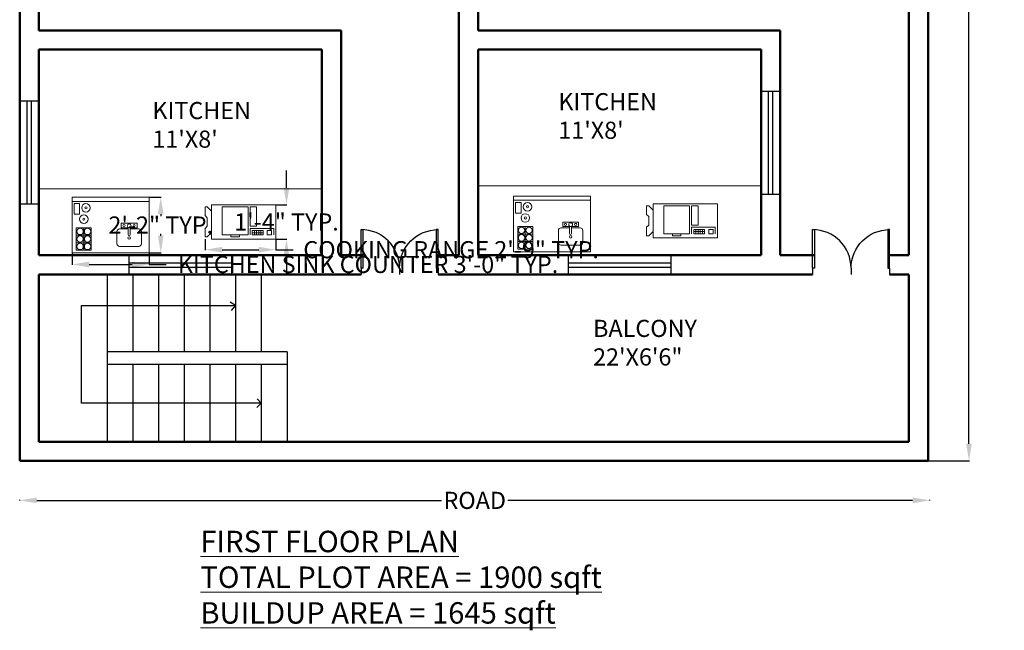
# Model space of a CAD drawing. Units: inches. Extents: x 179 to 2009, y 628 to 2084.
# Tile 3 of 5: x 766 to 1226, y 1391 to 1676. Entities that reach past the tile are written whole.
import ezdxf

# ---------------------------------------------------------------- set-up
doc = ezdxf.new("R2010")
doc.units = ezdxf.units.IN
doc.header["$MEASUREMENT"] = 0
for name, color, linetype, lineweight in [('A-ANNO-DIMS', 2, 'Continuous', 18), ('A-ANNO-TEXT', 7, 'Continuous', 18), ('A-DOOR', 3, 'Continuous', 25), ('A-FLOR-STRS', 6, 'Continuous', 25), ('A-FURN', 4, 'Continuous', 18), ('A-GLAZ', 2, 'Continuous', 25), ('A-WALL', 1, 'Continuous', 50)]:
    doc.layers.add(name, color=color, linetype=linetype, lineweight=lineweight)
doc.styles.get("Standard").update_dxf_attribs({"font": 'arial.ttf'})
doc.dimstyles.get("Standard").update_dxf_attribs({"dimtxt": 8, "dimasz": 8, "dimexe": 0.18, "dimexo": 0.0625, "dimgap": 0.09, "dimtad": 0, "dimtih": 1, "dimtoh": 1, "dimdec": 0, "dimzin": 0, "dimdsep": 46, "dimlunit": 3, "dimtxsty": 'Standard', "dimcen": 0.09, "dimadec": 0, "dimazin": 0, "dimtfac": 1, "dimtdec": 0, "dimtofl": 0, "dimtmove": 0, "dimatfit": 3, "dimfxl": 1, "dimtolj": 1, "dimtzin": 0, "dimarcsym": 0})

# ---------------------------------------------------------------- blocks, each defined once
blk = doc.blocks.new('*U4')
for p, q in [((0, 0), (0, -6)), ((36, 0), (36, -6))]:
    blk.add_line(p, q)
blk.add_lwpolyline([(0, 0), (0, 36), (1.75, 36), (1.75, 0)], close=True)
blk.add_arc((0, 0), 36, 0, 90)
blk = doc.blocks.new('Wet Bar')
for p, q in [((0, 0), (36, 0)), ((0, -26), (0, 0)), ((36, 0), (36, -26)), ((0, -2), (36, -2)), ((3.5, -3), (1, -3)), ((1, -3), (1, -8)), ((3.5, -8), (3.5, -3)), ((1, -8), (3.5, -8)), ((2, -14.25), (9, -14.25)), ((2, -24.75), (2, -14.25)), ((2, -17.75), (9, -17.75)), ((5.5, -14.25), (5.5, -24.75)), ((9, -14.25), (9, -24.75)), ((26.2, -17.55), (26.2, -14.1284)), ((27.1001, -17.55), (27.1001, -14.1284)), ((9, -21.25), (2, -21.25)), ((36, -26), (0, -26)), ((9, -24.75), (2, -24.75))]:
    blk.add_line(p, q)
for points in [[(26.2, -14.25), (22.95, -14.25), (22.95, -12.2), (26.75, -12.2)], [(26.7487, -12.2), (30.3501, -12.2), (30.3501, -14.25), (27.1001, -14.25)], [(20.95, -21.75), (20.95, -16.05)], [(22.15, -14.85), (26.2, -14.85)], [(27.1001, -14.85), (31.15, -14.85)], [(32.3501, -16.05), (32.3501, -21.75)], [(31.15, -22.95), (22.15, -22.95)]]:
    blk.add_lwpolyline(points)
for centre, radius in [((6.5, -5), 2), ((6.5, -5), 0.5), ((5.5, -10.25), 2), ((5.5, -10.25), 0.5), ((24.25, -13.25), 0.5), ((26.65, -13.35), 0.9), ((29, -13.25), 0.5), ((3.75, -16), 1.5), ((3.75, -19.5), 1.5), ((7.25, -16), 1.5), ((7.25, -19.5), 1.5), ((3.75, -23), 1.5), ((7.25, -23), 1.5), ((26.65, -19.05), 0.6)]:
    blk.add_circle(centre, radius)
for centre, radius, start, end in [((22.2251, -16.125), 1.2772, 93.36646, 176.6335), ((26.65, -17.55), 0.45, 180, 0), ((31.075, -16.125), 1.2772, 3.366461, 86.63354), ((22.2251, -21.675), 1.2772, 183.3665, 266.6335), ((31.075, -21.675), 1.2772, 273.3665, 356.6335)]:
    blk.add_arc(centre, radius, start, end)
blk = doc.blocks.new('Copy Machine')
for p, q in [((0, 0), (0, -16)), ((30, 0), (0, 0)), ((30, -16), (30, 0)), ((-3, -1), (-3, -5)), ((-2, -1), (-3, -1)), ((0, -3), (-2, -1)), ((5, -1), (5, -14)), ((17, -1), (5, -1)), ((17, -14), (17, -1)), ((18, -1), (18, -10)), ((21, -1), (18, -1)), ((21, -10), (21, -1)), ((-3, -5), (-2, -6)), ((-2, -10), (-2, -6)), ((-3, -11), (-2, -10)), ((-3, -15), (-3, -11)), ((0, -13), (-2, -15)), ((18, -10), (21, -10)), ((18, -14), (18, -11)), ((18, -11), (29, -11)), ((24, -12), (19, -12)), ((19, -12), (19, -14)), ((24, -13), (19, -13)), ((20, -12), (20, -14)), ((21, -14), (21, -12)), ((22, -12), (22, -14)), ((23, -14), (23, -12)), ((24, -14), (24, -12)), ((28, -12), (26, -12)), ((26, -12), (26, -14)), ((28, -14), (28, -12)), ((29, -11), (29, -14)), ((-2, -15), (-3, -15)), ((0, -16), (30, -16)), ((5, -14), (17, -14)), ((9, -14), (9, -15)), ((9, -15), (13, -15)), ((13, -15), (13, -14)), ((19, -14), (24, -14)), ((26, -14), (28, -14))]:
    blk.add_line(p, q)
blk = doc.blocks.new('*D18')
at = {"layer": 'A-ANNO-DIMS', "color": 0, "lineweight": -2, "transparency": 16777216}
for p, q in [((1190.56, 2043.18), (1209.72, 2043.18)), ((1209.54, 2035.18), (1209.54, 1760.86)), ((1209.54, 1478.18), (1209.54, 1752.51)), ((1190.56, 1470.18), (1209.72, 1470.18))]:
    blk.add_line(p, q, dxfattribs=at)
at = {"layer": 'A-ANNO-DIMS', "color": 0, "transparency": 16777216}
for points in [[(1208.21, 2035.18), (1210.88, 2035.18), (1209.54, 2043.18)], [(1208.21, 1478.18), (1210.88, 1478.18), (1209.54, 1470.18)]]:
    blk.add_solid(points, dxfattribs=at)
at = {"layer": 'Defpoints', "color": 0, "transparency": 16777216}
for p in [(1190.49, 2043.18), (1190.49, 1470.18), (1209.54, 1470.18)]:
    blk.add_point(p, dxfattribs=at)
at = {"layer": 'A-ANNO-DIMS', "color": 0, "transparency": 16777216, "insert": (1209.54, 1756.68), "char_height": 8, "attachment_point": 5}
blk.add_mtext('\\A1;47\'-9"', dxfattribs=at)
blk = doc.blocks.new('*D19')
at = {"layer": 'A-ANNO-DIMS', "color": 0, "lineweight": -2, "transparency": 16777216}
for p, q in [((766.49, 1451.68), (766.49, 1451.96)), ((774.49, 1451.78), (963.37, 1451.78)), ((1183.25, 1451.78), (994.37, 1451.78)), ((1191.25, 1451.68), (1191.25, 1451.96))]:
    blk.add_line(p, q, dxfattribs=at)
at = {"layer": 'A-ANNO-DIMS', "color": 0, "transparency": 16777216}
for points in [[(774.49, 1453.11), (774.49, 1450.44), (766.49, 1451.78)], [(1183.25, 1453.11), (1183.25, 1450.44), (1191.25, 1451.78)]]:
    blk.add_solid(points, dxfattribs=at)
at = {"layer": 'Defpoints', "color": 0, "transparency": 16777216}
for p in [(766.49, 1451.62), (1191.25, 1451.78), (1191.25, 1451.62)]:
    blk.add_point(p, dxfattribs=at)
at = {"layer": 'A-ANNO-DIMS', "color": 0, "transparency": 16777216, "insert": (978.87, 1451.78), "char_height": 8, "attachment_point": 5}
blk.add_mtext('\\A1;ROAD', dxfattribs=at)
blk = doc.blocks.new('*D53')
at = {"layer": 'A-ANNO-DIMS', "color": 0, "lineweight": -2, "transparency": 16777216}
for p, q in [((790.92, 1567.26), (790.92, 1561.74)), ((826.92, 1567.26), (826.92, 1561.74)), ((798.92, 1561.92), (818.92, 1561.92)), ((826.92, 1561.92), (834.92, 1561.92))]:
    blk.add_line(p, q, dxfattribs=at)
at = {"layer": 'A-ANNO-DIMS', "color": 0, "transparency": 16777216}
for points in [[(798.92, 1563.26), (798.92, 1560.59), (790.92, 1561.92)], [(818.92, 1563.26), (818.92, 1560.59), (826.92, 1561.92)]]:
    blk.add_solid(points, dxfattribs=at)
at = {"layer": 'Defpoints', "color": 0, "transparency": 16777216}
for p in [(790.92, 1567.32), (826.92, 1567.32), (826.92, 1561.92)]:
    blk.add_point(p, dxfattribs=at)
at = {"layer": 'A-ANNO-DIMS', "color": 0, "transparency": 16777216, "insert": (929.07, 1561.92), "char_height": 8, "attachment_point": 5}
blk.add_mtext('\\A1;KITCHEN SINK COUNTER 3\'-0" TYP.', dxfattribs=at)
blk = doc.blocks.new('*D54')
at = {"layer": 'A-ANNO-DIMS', "color": 0, "lineweight": -2, "transparency": 16777216}
for p, q in [((826.98, 1593.32), (832.5, 1593.32)), ((832.32, 1585.32), (832.32, 1584.43)), ((832.32, 1575.32), (832.32, 1576.22)), ((826.98, 1567.32), (832.5, 1567.32))]:
    blk.add_line(p, q, dxfattribs=at)
at = {"layer": 'A-ANNO-DIMS', "color": 0, "transparency": 16777216}
for points in [[(830.99, 1585.32), (833.66, 1585.32), (832.32, 1593.32)], [(830.99, 1575.32), (833.66, 1575.32), (832.32, 1567.32)]]:
    blk.add_solid(points, dxfattribs=at)
at = {"layer": 'Defpoints', "color": 0, "transparency": 16777216}
for p in [(826.92, 1593.32), (832.32, 1593.32), (826.92, 1567.32)]:
    blk.add_point(p, dxfattribs=at)
at = {"layer": 'A-ANNO-DIMS', "color": 0, "transparency": 16777216, "insert": (832.32, 1580.32), "char_height": 8, "attachment_point": 5}
blk.add_mtext('\\A1;2\'-2" TYP.', dxfattribs=at)
blk = doc.blocks.new('*D55')
at = {"layer": 'A-ANNO-DIMS', "color": 0, "lineweight": -2, "transparency": 16777216}
for p, q in [((853.06, 1573.69), (853.06, 1568.62)), ((886.06, 1573.69), (886.06, 1568.62)), ((861.06, 1568.8), (878.06, 1568.8)), ((886.06, 1568.8), (894.06, 1568.8))]:
    blk.add_line(p, q, dxfattribs=at)
at = {"layer": 'A-ANNO-DIMS', "color": 0, "transparency": 16777216}
for points in [[(861.06, 1570.14), (861.06, 1567.47), (853.06, 1568.8)], [(878.06, 1570.14), (878.06, 1567.47), (886.06, 1568.8)]]:
    blk.add_solid(points, dxfattribs=at)
at = {"layer": 'Defpoints', "color": 0, "transparency": 16777216}
for p in [(853.06, 1573.75), (886.06, 1573.75), (886.06, 1568.8)]:
    blk.add_point(p, dxfattribs=at)
at = {"layer": 'A-ANNO-DIMS', "color": 0, "transparency": 16777216, "insert": (967.85, 1568.8), "char_height": 8, "attachment_point": 5}
blk.add_mtext('\\A1;COOKING RANGE 2\'-9" TYP.', dxfattribs=at)
blk = doc.blocks.new('*D56')
at = {"layer": 'A-ANNO-DIMS', "color": 0, "lineweight": -2, "transparency": 16777216}
for p, q in [((891.01, 1597.75), (891.01, 1605.75)), ((886.12, 1589.75), (891.19, 1589.75)), ((886.12, 1573.75), (891.19, 1573.75)), ((891.01, 1565.75), (891.01, 1557.75))]:
    blk.add_line(p, q, dxfattribs=at)
at = {"layer": 'A-ANNO-DIMS', "color": 0, "transparency": 16777216}
for points in [[(889.67, 1597.75), (892.34, 1597.75), (891.01, 1589.75)], [(889.67, 1565.75), (892.34, 1565.75), (891.01, 1573.75)]]:
    blk.add_solid(points, dxfattribs=at)
at = {"layer": 'Defpoints', "color": 0, "transparency": 16777216}
for p in [(886.06, 1589.75), (891.01, 1589.75), (886.06, 1573.75)]:
    blk.add_point(p, dxfattribs=at)
at = {"layer": 'A-ANNO-DIMS', "color": 0, "transparency": 16777216, "insert": (891.01, 1581.75), "char_height": 8, "attachment_point": 5}
blk.add_mtext('\\A1;1\'-4" TYP.', dxfattribs=at)

msp = doc.modelspace()

# ---------------------------------------------------------------- linework, layer by layer
at = {"layer": 'A-FLOR-STRS'}
for p, q in [((807.27, 1557.18), (807.27, 1479.18)), ((819.27, 1557.18), (819.27, 1521.18)), ((831.27, 1557.18), (831.27, 1521.18)), ((843.27, 1557.18), (843.27, 1521.18)), ((855.27, 1557.18), (855.27, 1521.18)), ((867.27, 1557.18), (867.27, 1521.18)), ((879.27, 1557.18), (879.27, 1521.18)), ((867.27, 1542.77), (864.66, 1544.32)), ((795.41, 1497.18), (795.41, 1542.77)), ((795.41, 1542.77), (867.27, 1542.77)), ((867.27, 1542.77), (865.14, 1540.41)), ((891.27, 1521.18), (807.27, 1521.18)), ((891.27, 1521.18), (891.27, 1479.18)), ((891.27, 1515.18), (807.27, 1515.18)), ((819.27, 1515.18), (819.27, 1479.18)), ((831.27, 1515.18), (831.27, 1479.18)), ((843.27, 1515.18), (843.27, 1479.18)), ((855.27, 1515.18), (855.27, 1479.18)), ((867.27, 1515.18), (867.27, 1479.18)), ((879.27, 1515.18), (879.27, 1479.18)), ((879.27, 1497.18), (877.39, 1499.12)), ((879.27, 1497.18), (795.41, 1497.18)), ((879.27, 1497.18), (877.17, 1495.15))]:
    msp.add_line(p, q, dxfattribs=at)
at = {"layer": 'A-FURN'}
for p, q in [((775.49, 1597.18), (907.49, 1597.18)), ((1112.49, 1598.54), (980.49, 1598.54))]:
    msp.add_line(p, q, dxfattribs=at)
at = {"layer": 'A-GLAZ'}
for p, q in [((1115.99, 1594.68), (1115.99, 1642.68)), ((1117.99, 1594.68), (1117.99, 1642.68)), ((769.99, 1590.18), (769.99, 1638.18)), ((771.99, 1590.18), (771.99, 1638.18)), ((817.49, 1562.68), (865.49, 1562.68)), ((1022.49, 1562.68), (1070.49, 1562.68)), ((817.49, 1560.68), (865.49, 1560.68)), ((1022.49, 1560.68), (1070.49, 1560.68))]:
    msp.add_line(p, q, dxfattribs=at)
for points in [[(1121.49, 1594.68), (1121.49, 1642.68), (1112.49, 1642.68), (1112.49, 1594.68)], [(775.49, 1590.18), (775.49, 1638.18), (766.49, 1638.18), (766.49, 1590.18)], [(817.49, 1557.18), (865.49, 1557.18), (865.49, 1566.18), (817.49, 1566.18)], [(1022.49, 1557.18), (1070.49, 1557.18), (1070.49, 1566.18), (1022.49, 1566.18)]]:
    msp.add_lwpolyline(points, close=True, dxfattribs=at)
at = {"layer": 'A-WALL'}
for p, q in [((766.49, 2043.18), (766.49, 1470.18)), ((1190.49, 2043.18), (1190.49, 1470.18)), ((971.49, 1947.18), (971.49, 1566.18)), ((1181.49, 1947.18), (1181.49, 1566.18)), ((775.49, 1788.18), (775.49, 1671.18)), ((980.49, 1788.18), (980.49, 1671.18)), ((775.49, 1671.18), (916.49, 1671.18)), ((916.49, 1671.18), (916.49, 1566.18)), ((980.49, 1671.18), (1121.49, 1671.18)), ((1121.49, 1671.18), (1121.49, 1566.18)), ((775.49, 1662.18), (907.49, 1662.18)), ((775.49, 1662.18), (775.49, 1566.18)), ((907.49, 1662.18), (907.49, 1566.18)), ((980.49, 1662.18), (1112.49, 1662.18)), ((980.49, 1662.18), (980.49, 1566.18)), ((1112.49, 1662.18), (1112.49, 1566.18)), ((775.49, 1566.18), (907.49, 1566.18)), ((916.49, 1566.18), (926.66, 1566.18)), ((960.91, 1566.18), (971.49, 1566.18)), ((980.49, 1566.18), (1112.49, 1566.18)), ((1121.49, 1566.18), (1137.39, 1566.18)), ((1171.64, 1566.18), (1181.49, 1566.18)), ((775.49, 1557.18), (925.79, 1557.18)), ((775.49, 1557.18), (775.49, 1479.18)), ((961.79, 1557.18), (971.49, 1557.18)), ((971.49, 1557.18), (1136.52, 1557.18)), ((1172.52, 1557.18), (1181.49, 1557.18)), ((1181.49, 1557.18), (1181.49, 1479.18)), ((775.49, 1479.18), (971.49, 1479.18)), ((971.49, 1479.18), (1181.49, 1479.18)), ((766.49, 1470.18), (971.49, 1470.18)), ((971.49, 1470.18), (1190.49, 1470.18))]:
    msp.add_line(p, q, dxfattribs=at)

# ---------------------------------------------------------------- block references
at = {"layer": 'A-DOOR', "yscale": 0.5, "zscale": 0.5}
for p, xscale in [((925.79, 1560.18), 0.5), ((961.79, 1560.18), -0.5), ((1136.52, 1560.18), 0.5), ((1172.52, 1560.18), -0.5)]:
    msp.add_blockref('*U4', p, dxfattribs=dict(at, xscale=xscale))
at = {"layer": 'A-FURN'}
for name, p in [('Wet Bar', (790.92, 1593.32)), ('Wet Bar', (996.97, 1593.85)), ('Copy Machine', (1062.11, 1590.28)), ('Copy Machine', (856.06, 1589.75))]:
    msp.add_blockref(name, p, dxfattribs=at)

# ---------------------------------------------------------------- texts
at = {"layer": 'A-ANNO-TEXT', "attachment_point": 1}
for s, width, insert, char_height in [("KITCHEN\\P11'X8'", 129.4382, (1017.88, 1641.89), 8), ("KITCHEN\\P11'X8'", 129.4382, (828.42, 1637.75), 8), ('BALCONY\\P22\'X6\'6"', 129.4382, (1034.1, 1536.07), 8), ('{\\fArial|b1|i0|c0|p34;\\LFIRST FLOOR PLAN\\PTOTAL PLOT AREA = 1900 sqft\\PBUILDUP AREA = 1645 sqft}', 261.1575, (850.81, 1437.59), 10)]:
    msp.add_mtext_dynamic_manual_height_columns(s, width=width, gutter_width=1, heights=[0], dxfattribs=dict(at, insert=insert, char_height=char_height))

# ---------------------------------------------------------------- dimensions: what is measured, and where the dimension line sits
at = {"layer": 'A-ANNO-DIMS'}
dim = msp.add_linear_dim(base=(1209.54, 1470.18), p1=(1190.49, 2043.18), p2=(1190.49, 1470.18), angle=90, dimstyle='Standard', override={"dimclrd": 0, "dimclre": 0, "dimclrt": 0}, dxfattribs=at)
dim.commit()
dim.dimension.update_dxf_attribs({"geometry": '*D18', "text_midpoint": (1209.54, 1756.68)})
for base, p1, p2, picture, middle in [((891.01, 1589.75), (886.06, 1573.75), (886.06, 1589.75), '*D56', (891.01, 1581.75)), ((832.32, 1593.32), (826.92, 1567.32), (826.92, 1593.32), '*D54', (832.32, 1580.32))]:
    dim = msp.add_linear_dim(base=base, p1=p1, p2=p2, angle=90, text='<> TYP.', dimstyle='Standard', override={"dimdec": 1, "dimrnd": 0, "dimzin": 1, "dimlunit": 4, "dimfrac": 2}, dxfattribs=at)
    dim.commit()
    dim.dimension.update_dxf_attribs({"geometry": picture, "text_midpoint": middle})
for base, p1, p2, text, override, picture, middle in [((826.92, 1561.92), (790.92, 1567.32), (826.92, 1567.32), 'KITCHEN SINK COUNTER <> TYP.', {"dimdec": 1, "dimrnd": 0, "dimzin": 1, "dimlunit": 4, "dimfrac": 2}, '*D53', (929.07, 1561.92)), ((886.06, 1568.8), (853.06, 1573.75), (886.06, 1573.75), 'COOKING RANGE <> TYP.', {"dimdec": 1, "dimrnd": 0, "dimzin": 1, "dimlunit": 4, "dimfrac": 2}, '*D55', (967.85, 1568.8)), ((1191.25, 1451.78), (766.49, 1451.62), (1191.25, 1451.62), 'ROAD', {"dimclrd": 0, "dimclre": 0, "dimclrt": 0}, '*D19', (978.87, 1451.78))]:
    dim = msp.add_linear_dim(base=base, p1=p1, p2=p2, text=text, dimstyle='Standard', override=override, dxfattribs=at)
    dim.commit()
    dim.dimension.update_dxf_attribs({"geometry": picture, "text_midpoint": middle})

doc.saveas('drawing.dxf')
